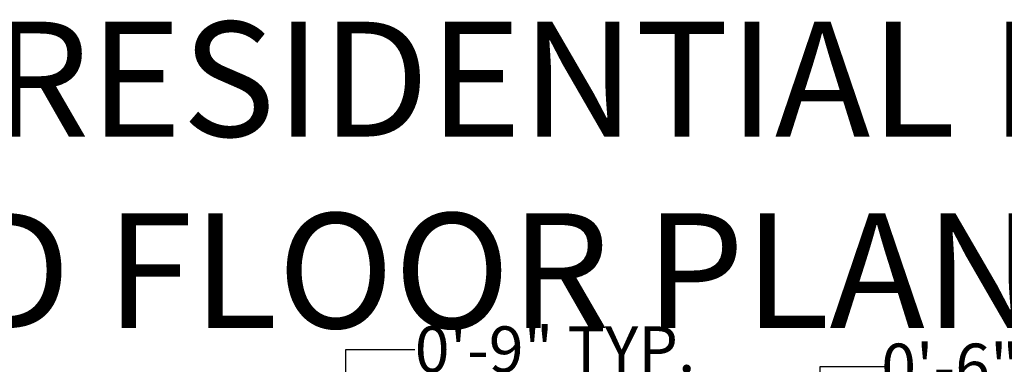
# Model space of a CAD drawing. Units: inches. Extents: x 2838 to 4029, y 1041 to 1915.
# Tile 15 of 16: x 3250 to 3764, y 1735 to 1915. Entities that reach past the tile are written whole.
import ezdxf

# ---------------------------------------------------------------- set-up
doc = ezdxf.new("R2010")
doc.units = ezdxf.units.IN
doc.header["$MEASUREMENT"] = 0
doc.layers.add('A-ANNO-DIMS', color=2, linetype='Continuous', lineweight=18)
doc.layers.add('A-ANNO-TEXT', color=7, linetype='Continuous', lineweight=18)
doc.styles.get("Standard").update_dxf_attribs({"font": 'arial.ttf'})
doc.dimstyles.get("Standard").update_dxf_attribs({"dimtxt": 24, "dimasz": 36, "dimexe": 0.18, "dimexo": 0.0625, "dimgap": 0.09, "dimtad": 0, "dimtih": 1, "dimtoh": 1, "dimdec": 0, "dimzin": 0, "dimdsep": 46, "dimlunit": 3, "dimtxsty": 'Standard', "dimcen": 0.09, "dimadec": 0, "dimazin": 0, "dimtfac": 1, "dimtdec": 0, "dimtofl": 0, "dimtmove": 0, "dimatfit": 3, "dimfxl": 1, "dimtolj": 1, "dimtzin": 0, "dimarcsym": 0})

# ---------------------------------------------------------------- blocks, each defined once
blk = doc.blocks.new('*D39')
at = {"layer": 'A-ANNO-DIMS', "color": 0, "lineweight": -2, "transparency": 16777216}
for p, q in [((3391.52, 1678.5), (3355.52, 1678.5)), ((3427.52, 1671.36), (3427.52, 1678.68)), ((3475.52, 1671.36), (3475.52, 1678.68)), ((3511.52, 1678.5), (3547.52, 1678.5))]:
    blk.add_line(p, q, dxfattribs=at)
at = {"layer": 'A-ANNO-DIMS', "color": 0, "transparency": 16777216}
for points in [[(3391.52, 1684.5), (3391.52, 1672.5), (3427.52, 1678.5)], [(3511.52, 1684.5), (3511.52, 1672.5), (3475.52, 1678.5)]]:
    blk.add_solid(points, dxfattribs=at)
at = {"layer": 'Defpoints', "color": 0, "transparency": 16777216}
for p in [(3475.52, 1678.5), (3427.52, 1671.3), (3475.52, 1671.3)]:
    blk.add_point(p, dxfattribs=at)
at = {"layer": 'A-ANNO-DIMS', "color": 0, "transparency": 16777216, "insert": (3732.24, 1678.5), "char_height": 24, "attachment_point": 5}
blk.add_mtext('\\A1;VENT BLOCK 4\'-0" TYP.', dxfattribs=at)
blk = doc.blocks.new('*D40')
at = {"layer": 'A-ANNO-DIMS', "color": 0, "lineweight": -2, "transparency": 16777216}
for p, q in [((3420.32, 1707.3), (3420.32, 1743.3)), ((3420.32, 1743.3), (3456.32, 1743.3)), ((3427.46, 1671.3), (3420.14, 1671.3)), ((3427.46, 1662.3), (3420.14, 1662.3)), ((3420.32, 1626.3), (3420.32, 1590.3))]:
    blk.add_line(p, q, dxfattribs=at)
at = {"layer": 'A-ANNO-DIMS', "color": 0, "transparency": 16777216}
for points in [[(3414.32, 1707.3), (3426.32, 1707.3), (3420.32, 1671.3)], [(3414.32, 1626.3), (3426.32, 1626.3), (3420.32, 1662.3)]]:
    blk.add_solid(points, dxfattribs=at)
at = {"layer": 'Defpoints', "color": 0, "transparency": 16777216}
for p in [(3420.32, 1671.3), (3427.52, 1671.3), (3427.52, 1662.3)]:
    blk.add_point(p, dxfattribs=at)
at = {"layer": 'A-ANNO-DIMS', "color": 0, "transparency": 16777216, "insert": (3529.56, 1743.3), "char_height": 24, "attachment_point": 5}
blk.add_mtext('\\A1;0\'-9" TYP.', dxfattribs=at)
blk = doc.blocks.new('*D73')
at = {"layer": 'A-ANNO-DIMS', "color": 0, "lineweight": -2, "transparency": 16777216}
for p, q in [((3425.038746, 1711.522346), (3389.038746, 1711.522346)), ((3461.038746, 1200.359846), (3461.038746, 1711.702346)), ((3618.731626, 1200.359846), (3618.731626, 1711.702346)), ((3654.731626, 1711.522346), (3690.731626, 1711.522346))]:
    blk.add_line(p, q, dxfattribs=at)
at = {"layer": 'A-ANNO-DIMS', "color": 0, "transparency": 16777216}
for points in [[(3425.038746, 1717.522346), (3425.038746, 1705.522346), (3461.038746, 1711.522346)], [(3654.731626, 1717.522346), (3654.731626, 1705.522346), (3618.731626, 1711.522346)]]:
    blk.add_solid(points, dxfattribs=at)
at = {"layer": 'Defpoints', "color": 0, "transparency": 16777216}
for p in [(3618.731626, 1711.522346), (3461.038746, 1200.297346), (3618.731626, 1200.297346)]:
    blk.add_point(p, dxfattribs=at)
at = {"layer": 'A-ANNO-DIMS', "color": 0, "transparency": 16777216, "insert": (3539.885186, 1711.522346), "char_height": 24, "attachment_point": 5}
blk.add_mtext('\\A1;13\'-1 1/2"', dxfattribs=at)
blk = doc.blocks.new('*D79')
at = {"layer": 'A-ANNO-DIMS', "color": 0, "lineweight": -2, "transparency": 16777216}
for p, q in [((3379.05, 1400.64), (3379.05, 1711.7)), ((3415.05, 1711.52), (3418.63, 1711.52)), ((3454.63, 1398.31), (3454.63, 1711.7)), ((3454.63, 1711.52), (3490.63, 1711.52))]:
    blk.add_line(p, q, dxfattribs=at)
at = {"layer": 'A-ANNO-DIMS', "color": 0, "transparency": 16777216}
for points in [[(3415.05, 1717.52), (3415.05, 1705.52), (3379.05, 1711.52)], [(3418.63, 1717.52), (3418.63, 1705.52), (3454.63, 1711.52)]]:
    blk.add_solid(points, dxfattribs=at)
at = {"layer": 'Defpoints', "color": 0, "transparency": 16777216}
for p in [(3454.63, 1711.52), (3379.05, 1400.57), (3454.63, 1398.25)]:
    blk.add_point(p, dxfattribs=at)
at = {"layer": 'A-ANNO-DIMS', "color": 0, "transparency": 16777216, "insert": (3550.65, 1711.52), "char_height": 24, "attachment_point": 5}
blk.add_mtext('\\A1;6\'-3 1/2"', dxfattribs=at)
blk = doc.blocks.new('*D96')
at = {"layer": 'A-ANNO-DIMS', "color": 0, "lineweight": -2, "transparency": 16777216}
for p, q in [((3462.73, 1711.52), (3426.73, 1711.52)), ((3498.73, 1662.36), (3498.73, 1711.7)), ((3546.42, 1662.36), (3546.42, 1711.7)), ((3582.42, 1711.52), (3618.42, 1711.52))]:
    blk.add_line(p, q, dxfattribs=at)
at = {"layer": 'A-ANNO-DIMS', "color": 0, "transparency": 16777216}
for points in [[(3462.73, 1717.52), (3462.73, 1705.52), (3498.73, 1711.52)], [(3582.42, 1717.52), (3582.42, 1705.52), (3546.42, 1711.52)]]:
    blk.add_solid(points, dxfattribs=at)
at = {"layer": 'Defpoints', "color": 0, "transparency": 16777216}
for p in [(3546.42, 1711.52), (3498.73, 1662.3), (3546.42, 1662.3)]:
    blk.add_point(p, dxfattribs=at)
at = {"layer": 'A-ANNO-DIMS', "color": 0, "transparency": 16777216, "insert": (3687.68, 1711.52), "char_height": 24, "attachment_point": 5}
blk.add_mtext('\\A1;3\'-11 1/2"', dxfattribs=at)
blk = doc.blocks.new('*D102')
at = {"layer": 'A-ANNO-DIMS', "color": 0, "lineweight": -2, "transparency": 16777216}
for p, q in [((3667.96, 1698.3), (3667.96, 1734.3)), ((3667.96, 1734.3), (3703.96, 1734.3)), ((3489.79, 1662.3), (3668.14, 1662.3)), ((3489.79, 1656.41), (3668.14, 1656.41)), ((3667.96, 1620.41), (3667.96, 1584.41))]:
    blk.add_line(p, q, dxfattribs=at)
at = {"layer": 'A-ANNO-DIMS', "color": 0, "transparency": 16777216}
for points in [[(3661.96, 1698.3), (3673.96, 1698.3), (3667.96, 1662.3)], [(3661.96, 1620.41), (3673.96, 1620.41), (3667.96, 1656.41)]]:
    blk.add_solid(points, dxfattribs=at)
at = {"layer": 'Defpoints', "color": 0, "transparency": 16777216}
for p in [(3489.73, 1662.3), (3667.96, 1662.3), (3489.73, 1656.41)]:
    blk.add_point(p, dxfattribs=at)
at = {"layer": 'A-ANNO-DIMS', "color": 0, "transparency": 16777216, "insert": (3735.95, 1734.3), "char_height": 24, "attachment_point": 5}
blk.add_mtext('\\A1;0\'-6"', dxfattribs=at)
blk = doc.blocks.new('*D105')
at = {"layer": 'A-ANNO-DIMS', "color": 0, "lineweight": -2, "transparency": 16777216}
for p, q in [((3578.46, 1711.52), (3542.46, 1711.52)), ((3614.46, 1472.42), (3614.46, 1711.7)), ((3618.73, 1469.91), (3618.73, 1711.7)), ((3654.73, 1711.52), (3690.73, 1711.52))]:
    blk.add_line(p, q, dxfattribs=at)
at = {"layer": 'A-ANNO-DIMS', "color": 0, "transparency": 16777216}
for points in [[(3578.46, 1717.52), (3578.46, 1705.52), (3614.46, 1711.52)], [(3654.73, 1717.52), (3654.73, 1705.52), (3618.73, 1711.52)]]:
    blk.add_solid(points, dxfattribs=at)
at = {"layer": 'Defpoints', "color": 0, "transparency": 16777216}
for p in [(3618.73, 1711.52), (3614.46, 1472.36), (3618.73, 1469.85)]:
    blk.add_point(p, dxfattribs=at)
at = {"layer": 'A-ANNO-DIMS', "color": 0, "transparency": 16777216, "insert": (3750.68, 1711.52), "char_height": 24, "attachment_point": 5}
blk.add_mtext('\\A1;0\'-4 1/2"', dxfattribs=at)

msp = doc.modelspace()

# ---------------------------------------------------------------- texts
at = {"layer": 'A-ANNO-TEXT', "insert": (3004.58, 1914.43), "char_height": 60, "attachment_point": 1}
msp.add_mtext_dynamic_manual_height_columns('2BHK RESIDENTIAL HOUSE \\P------2D FLOOR PLAN------', width=1981.8988, gutter_width=1, heights=[0], dxfattribs=at)

# ---------------------------------------------------------------- dimensions: what is measured, and where the dimension line sits
at = {"layer": 'A-ANNO-DIMS'}
dim = msp.add_linear_dim(base=(3420.32, 1671.3), p1=(3427.52, 1662.3), p2=(3427.52, 1671.3), angle=90, text='<> TYP.', dimstyle='Standard', override={"dimdec": 1, "dimlfac": 1, "dimrnd": 0, "dimzin": 1, "dimdsep": 46, "dimlunit": 4, "dimfrac": 2}, dxfattribs=at)
dim.commit()
dim.dimension.update_dxf_attribs({"geometry": '*D40', "text_midpoint": (3529.56, 1743.3)})
dim = msp.add_linear_dim(base=(3475.52, 1678.5), p1=(3427.52, 1671.3), p2=(3475.52, 1671.3), text='VENT BLOCK <> TYP.', dimstyle='Standard', override={"dimdec": 1, "dimlfac": 1, "dimrnd": 0, "dimzin": 1, "dimdsep": 46, "dimlunit": 4, "dimfrac": 2}, dxfattribs=at)
dim.commit()
dim.dimension.update_dxf_attribs({"geometry": '*D39', "text_midpoint": (3732.24, 1678.5)})
for base, p1, p2, picture, middle in [((3454.63, 1711.52), (3379.05, 1400.57), (3454.63, 1398.25), '*D79', (3550.65, 1711.52)), ((3618.73, 1711.52), (3461.04, 1200.3), (3618.73, 1200.3), '*D73', (3539.89, 1711.52)), ((3546.42, 1711.52), (3498.73, 1662.3), (3546.42, 1662.3), '*D96', (3687.68, 1711.52)), ((3618.73, 1711.52), (3614.46, 1472.36), (3618.73, 1469.85), '*D105', (3750.68, 1711.52))]:
    dim = msp.add_linear_dim(base=base, p1=p1, p2=p2, dimstyle='Standard', override={"dimdec": 1, "dimlfac": 1, "dimrnd": 0, "dimzin": 1, "dimdsep": 46, "dimlunit": 4, "dimfrac": 2}, dxfattribs=at)
    dim.commit()
    dim.dimension.update_dxf_attribs({"geometry": picture, "text_midpoint": middle})
dim = msp.add_linear_dim(base=(3667.96, 1662.3), p1=(3489.73, 1656.41), p2=(3489.73, 1662.3), angle=90, dimstyle='Standard', override={"dimdec": 1, "dimlfac": 1, "dimrnd": 0, "dimzin": 1, "dimdsep": 46, "dimlunit": 4, "dimfrac": 2}, dxfattribs=at)
dim.commit()
dim.dimension.update_dxf_attribs({"geometry": '*D102', "text_midpoint": (3735.95, 1734.3)})

doc.saveas('drawing.dxf')
